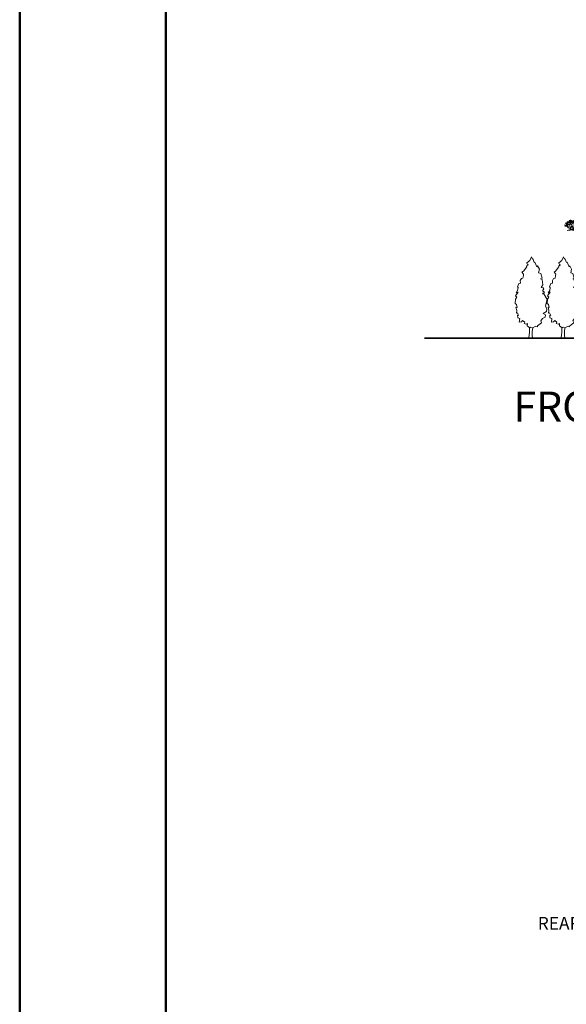
# Model space of a CAD drawing. Units: inches. Extents: x -1080 to 1950, y -1929 to 857.
# Tile 2 of 16: x -1080 to -622, y -550 to 276. Entities that reach past the tile are written whole.
import ezdxf

# ---------------------------------------------------------------- set-up
doc = ezdxf.new("R2010")
doc.units = ezdxf.units.IN
doc.header["$MEASUREMENT"] = 0
for name, color, linetype, lineweight in [('A-ANNO-TEXT', 7, 'Continuous', 25), ('A-ANNO-TTLB', 7, 'Continuous', 50), ('A-ELEV', 7, 'Continuous', 35), ('L-PLNT', 82, 'Continuous', 13)]:
    doc.layers.add(name, color=color, linetype=linetype, lineweight=lineweight)
doc.styles.get("Standard").update_dxf_attribs({"font": 'arial.ttf'})

# ---------------------------------------------------------------- blocks, each defined once
blk = doc.blocks.new('*U5')
blk.add_lwpolyline([(-2.754, 191.699), (-6.78, 182.851), (-13.682, 176.953), (-11.956, 173.266), (-9.656, 172.529), (-14.257, 170.317), (-13.682, 167.368), (-21.733, 157.783), (-25.184, 154.834), (-21.158, 150.41), (-21.733, 147.461), (-22.884, 140.825), (-26.334, 140.087), (-29.21, 134.926), (-28.635, 129.028), (-32.661, 128.291), (-36.111, 120.18), (-34.386, 118.706), (-35.536, 111.333), (-38.987, 106.171), (-34.386, 107.646), (-40.712, 98.798), (-37.261, 95.849), (-40.712, 90.688), (-41.287, 80.366), (-38.412, 78.154), (-36.686, 70.781), (-39.562, 71.518), (-37.261, 64.145), (-38.412, 57.509), (-36.111, 58.247), (-33.236, 52.348), (-35.536, 53.086), (-34.961, 46.45), (-30.36, 44.975), (-31.51, 36.128), (-26.334, 36.865), (-23.459, 39.814), (-18.283, 36.128), (-20.008, 33.178), (-14.832, 31.704), (-11.956, 33.178), (-12.531, 27.28), (-6.205, 22.856), (-3.905, 24.331), (0.121, 22.856), (8.173, 26.543), (11.624, 25.068), (12.199, 27.28), (21.4, 34.653), (19.675, 39.077), (23.701, 44.975), (30.027, 47.924), (30.602, 53.823), (25.426, 56.772), (32.903, 61.196), (34.053, 67.094), (30.602, 75.205), (34.628, 89.951), (26.576, 103.222), (23.701, 103.222), (28.302, 107.646), (23.701, 110.595), (26.576, 115.756), (25.426, 117.968), (20.825, 118.706), (24.276, 124.604), (22.551, 137.876), (19.1, 139.35), (22.551, 140.825), (19.675, 151.884), (14.499, 153.359), (16.224, 162.207), (12.199, 170.317), (10.473, 167.368), (5.872, 179.165), (4.147, 177.69), (0.696, 187.275), (-0.454, 185.8)], close=True)
for points in [[(-6.813, 23.669), (-6.813, 11.669), (-8.627, 0)], [(0.387, 23.669), (-0.576, 13.271), (-0.576, 3.686), (0, 0)]]:
    blk.add_lwpolyline(points)
blk = doc.blocks.new('*U6')
for p, q in [((-316.7634, 502.285), (-327.6092, 559.9176)), ((-290.3982, 464.5406), (-265.6078, 577.8246)), ((-207.264, 451.104), (-268.224, 548.64)), ((-240.792, 502.285), (-228.3968, 573.8368)), ((-134.112, 487.68), (-97.536, 548.64)), ((-85.7758, 472.4908), (-73.3552, 548.005)), ((-12.9032, 555.9552), (-2.0574, 522.1732)), ((1.0414, 526.1356), (35.1536, 559.9176)), ((2.5908, 542.036), (21.209, 555.9552)), ((-451.104, 219.456), (-601.0402, 303.8094)), ((-451.104, 219.456), (-587.4512, 234.2388)), ((-463.296, 280.416), (-552.577, 423.037)), ((-463.296, 280.416), (-512.064, 292.608)), ((-329.184, 316.992), (-499.872, 414.528)), ((-353.568, 316.992), (-487.68, 377.952)), ((-426.72, 414.528), (-475.488, 475.488)), ((-402.336, 207.264), (-463.296, 280.416)), ((-414.528, 182.88), (-463.296, 182.88)), ((-377.952, 463.296), (-451.104, 487.68)), ((-426.72, 316.992), (-451.104, 329.184)), ((-377.952, 146.304), (-451.104, 219.456)), ((-402.336, 12.192), (-451.104, 0)), ((-426.72, 414.528), (-390.144, 499.872)), ((-426.72, 316.992), (-426.72, 414.528)), ((-402.336, 207.264), (-426.72, 316.992)), ((-377.952, 146.304), (-402.336, 207.264)), ((-341.376, 12.192), (-402.336, 12.192)), ((-377.952, 463.296), (-329.184, 524.256)), ((-207.264, 304.8), (-377.952, 463.296)), ((-329.184, 121.92), (-377.952, 146.304)), ((-329.184, 316.992), (-353.568, 316.992)), ((-243.84, 24.384), (-341.376, 12.192)), ((-338.455, 424.7896), (-290.3982, 464.5406)), ((-329.184, 316.992), (-207.264, 451.104)), ((-268.224, 109.728), (-329.184, 316.992)), ((-292.608, 60.96), (-329.184, 121.92)), ((-243.84, 24.384), (-329.184, 0)), ((-296.5958, 484.4034), (-316.7634, 502.285)), ((-286.512, 498.3226), (-307.4416, 538.0736)), ((-305.8922, 396.9512), (-302.7934, 478.4344)), ((-304.3428, 426.7708), (-268.7066, 458.5716)), ((-302.7934, 478.4344), (-270.256, 518.1854)), ((-219.456, 24.384), (-292.608, 60.96)), ((-268.7066, 458.5716), (-250.0884, 500.3038)), ((-268.224, 109.728), (-219.456, 195.072)), ((-219.456, 48.768), (-268.224, 109.728)), ((-243.84, 24.384), (-195.072, 24.384)), ((-182.88, 499.872), (-219.456, 512.064)), ((-219.456, 195.072), (-207.264, 304.8)), ((-219.456, 24.384), (-109.728, 73.152)), ((-219.456, 24.384), (-158.496, 73.152)), ((-219.456, 24.384), (-219.456, 48.768)), ((-219.456, 24.384), (-73.152, 24.384)), ((-207.264, 451.104), (-134.112, 487.68)), ((-195.072, 316.992), (-182.88, 377.952)), ((-170.688, 219.456), (-195.072, 316.992)), ((-195.072, 24.384), (-158.496, 12.192)), ((-182.88, 499.872), (-158.496, 536.448)), ((-121.92, 414.528), (-182.88, 499.872)), ((-182.88, 377.952), (-97.536, 426.72)), ((-146.304, 134.112), (-170.688, 219.456)), ((-158.496, 73.152), (-146.304, 134.112)), ((-158.496, 12.192), (-85.344, 0)), ((-129.1844, 450.6214), (-140.0302, 542.036)), ((-85.7758, 389.001), (-129.1844, 452.6026)), ((-73.152, 329.184), (-109.728, 499.872)), ((-109.728, 73.152), (-48.768, 243.84)), ((-97.536, 426.72), (-24.384, 524.256)), ((-70.2564, 426.7708), (-85.7758, 472.4908)), ((-85.344, 134.112), (-73.152, 329.184)), ((-73.152, 402.336), (-60.96, 512.064)), ((-24.384, 268.224), (-73.152, 402.336)), ((-73.152, 24.384), (0, 0)), ((-48.768, 243.84), (24.384, 304.8)), ((-12.192, 274.32), (8.7884, 335.3562)), ((-5.1562, 486.3846), (2.5908, 542.036)), ((8.7884, 335.3562), (-5.1562, 486.3846)), ((-3.6068, 492.3536), (14.986, 518.1854)), ((-0.508, 508.254), (22.7584, 536.067)), ((8.7884, 335.3562), (33.6042, 412.8516)), ((24.384, 304.8), (36.576, 390.144)), ((24.384, 304.8), (73.152, 377.952)), ((33.6042, 412.8516), (92.5068, 464.5406)), ((36.576, 390.144), (73.152, 438.912)), ((48.768, 341.376), (60.96, 390.144)), ((60.96, 390.144), (85.344, 414.528))]:
    blk.add_line(p, q)

msp = doc.modelspace()

# ---------------------------------------------------------------- linework, layer by layer
at = {"layer": 'A-ANNO-TTLB'}
for points in [[(-1080.09, 856.52), (1950.41, 856.52), (1950.41, -1928.98), (-1080.09, -1928.98)], [(-957.59, 743.52), (1813.41, 743.52), (1813.41, -1770.48), (-957.59, -1770.48)]]:
    msp.add_lwpolyline(points, close=True, dxfattribs=at)
at = {"layer": 'A-ELEV'}
for p in [(-148.56, 9.02), (-129.68, 9.02)]:
    msp.add_line(p, (-740.58, 9.02), dxfattribs=at)

# ---------------------------------------------------------------- block references
at = {"layer": 'L-PLNT'}
for name, p, xscale, yscale, zscale in [('*U6', (-613.89, 99.47), 0.0152219259934872, 0.0152219259934872, 0.0152219259934872), ('*U5', (-649.92, 9.75), 0.3528399638811642, 0.3528399638811642, 0.3528399638811642), ('*U5', (-622.96, 9.75), 0.3528399638811642, 0.3528399638811642, 0.3528399638811642)]:
    msp.add_blockref(name, p, dxfattribs=dict(at, xscale=xscale, yscale=yscale, zscale=zscale))

# ---------------------------------------------------------------- texts
at = {"layer": 'A-ANNO-TEXT'}
for s, height, p in [('FRONT   ELEVATION - MAIN   ACADEMIC   AND   INNOVATION   COMPLEX', 25.272, (-665.96, -61.01)), ('REAR  SERVICE   ROOM', 10.6643, (-645.54, -487.22))]:
    msp.add_text(s, height=height, dxfattribs=at).set_placement(p)

doc.saveas('drawing.dxf')
